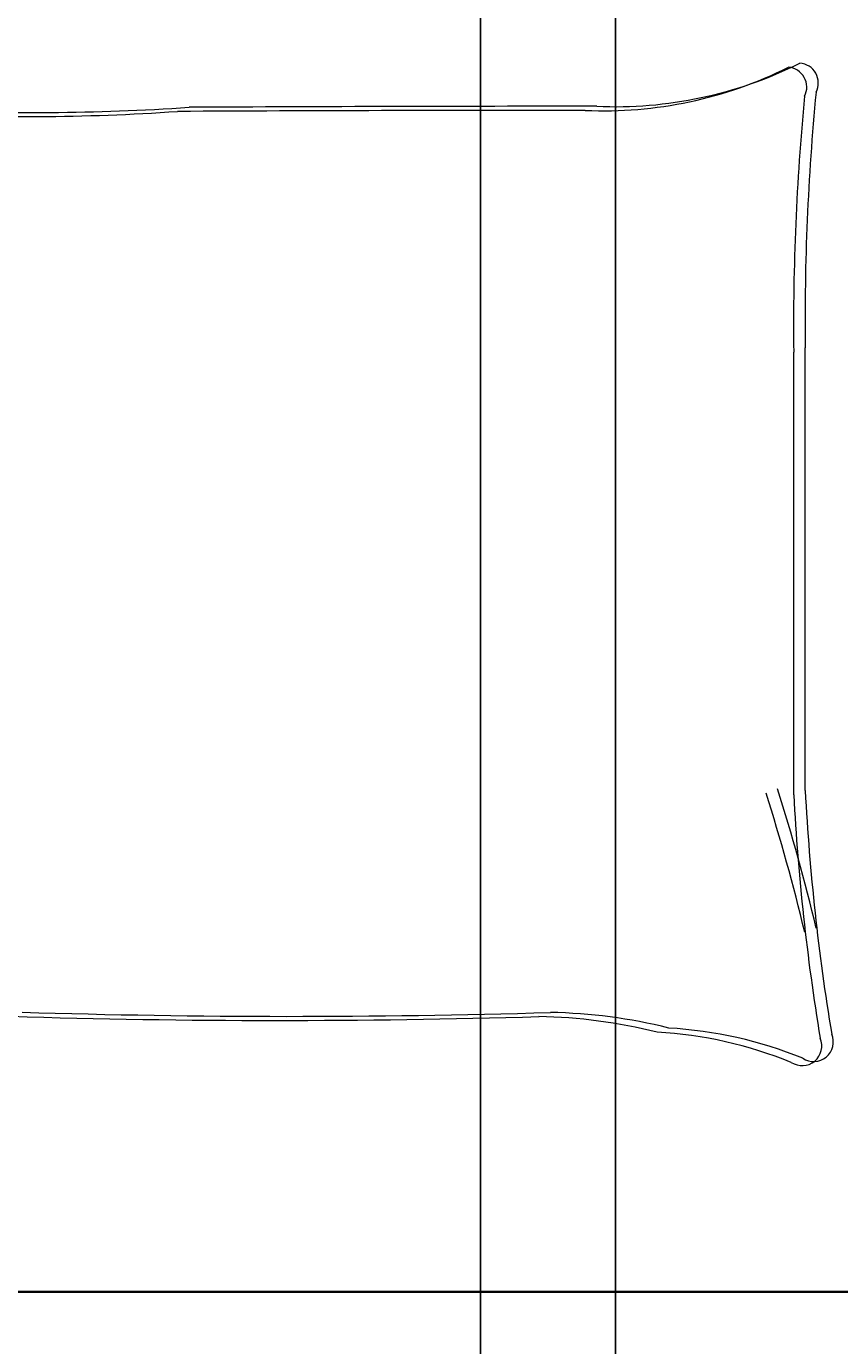
# Model space of a CAD drawing. Units: inches. Extents: x 1088 to 1703, y 668 to 1875.
# Tile 25 of 45: x 1484 to 1539, y 1416 to 1504. Entities that reach past the tile are written whole.
import ezdxf

# ---------------------------------------------------------------- set-up
doc = ezdxf.new("R2010")
doc.units = ezdxf.units.IN
for name, color, linetype, lineweight in [('A-ANNO-DIMS', 2, 'Continuous', 18), ('A-FURN', 8, 'Continuous', 13), ('A-WALL', 7, 'Continuous', 35)]:
    doc.layers.add(name, color=color, linetype=linetype, lineweight=lineweight)
doc.styles.get("Standard").update_dxf_attribs({"font": 'arial.ttf'})
doc.dimstyles.get("Standard").update_dxf_attribs({"dimtxt": 0.18, "dimasz": 0.18, "dimexe": 0.18, "dimexo": 0.0625, "dimgap": 0.09, "dimtad": 0, "dimtih": 1, "dimtoh": 1, "dimdec": 4, "dimzin": 0, "dimdsep": 46, "dimtxsty": 'Standard', "dimcen": 0.09, "dimadec": 0, "dimazin": 0, "dimtfac": 1, "dimtdec": 4, "dimtofl": 0, "dimtmove": 0, "dimatfit": 3, "dimfxl": 1, "dimtolj": 1, "dimtzin": 0, "dimarcsym": 0})

# ---------------------------------------------------------------- blocks, each defined once
blk = doc.blocks.new('BED-DOUBLE')
for p, q in [((95.003, 18.059), (95.003, 47.568)), ((95.77, 18.333), (95.77, 47.841))]:
    blk.add_line(p, q)
for centre, radius, start, end in [((82.321, 91.302), 27.652, 267.47136, 296.46809), ((83.088, 91.576), 27.652, 267.47136, 296.46809), ((94.554, 65.23), 1.322, 332.65876, 86.02002), ((95.32, 65.504), 1.322, 332.65876, 86.02002), ((254.489, 49.336), 159.496, 174.4998, 180.63509), ((255.256, 49.609), 159.496, 174.4998, 180.63509), ((43.537, 218.511), 155.251, 266.97912, 273.83645), ((44.303, 218.785), 155.251, 266.97912, 273.83645), ((81.308, -5405.342), 5469.019, 90.002168, 90.286887), ((82.075, -5405.068), 5469.019, 90.002168, 90.286887), ((-28.427, -20.646), 127.629, 13.38322, 17.70533), ((-27.661, -20.372), 127.629, 13.38322, 17.70533), ((240.775, 25.688), 145.971, 182.99578, 189.40907), ((241.542, 25.962), 145.971, 182.99578, 189.40907), ((61.445, 581.507), 578.221, 268.227709, 271.718541), ((78.111, -31.975), 35.527, 76.06484, 88.91125), ((60.679, 581.233), 578.221, 268.227709, 271.718541), ((77.344, -32.248), 35.527, 76.06484, 88.91125), ((84.25, -25.966), 28.247, 67.97508, 86.652), ((85.017, -25.693), 28.247, 67.97508, 86.652), ((95.57, 1.304), 1.306, 236.17358, 23.47814), ((96.337, 1.578), 1.306, 236.17358, 23.47814)]:
    blk.add_arc(centre, radius, start, end)
blk = doc.blocks.new('*D33')
at = {"layer": 'A-ANNO-DIMS', "color": 0, "lineweight": -2, "transparency": 16777216}
for p, q in [((1514.595, 1355.648), (1514.595, 1857.788)), ((1514.775, 1857.608), (1518.946, 1857.608)), ((1523.415, 1857.608), (1519.244, 1857.608)), ((1523.595, 1331.121), (1523.595, 1857.788))]:
    blk.add_line(p, q, dxfattribs=at)
at = {"layer": 'A-ANNO-DIMS', "color": 0, "transparency": 16777216}
for points in [[(1514.775, 1857.638), (1514.775, 1857.578), (1514.595, 1857.608)], [(1523.415, 1857.638), (1523.415, 1857.578), (1523.595, 1857.608)]]:
    blk.add_solid(points, dxfattribs=at)
at = {"layer": 'Defpoints', "color": 0, "transparency": 16777216}
for p in [(1523.595, 1857.608), (1514.595, 1355.585), (1523.595, 1331.058)]:
    blk.add_point(p, dxfattribs=at)
at = {"layer": 'A-ANNO-DIMS', "color": 0, "transparency": 16777216, "insert": (1519.095, 1857.608), "char_height": 0.18, "attachment_point": 5}
blk.add_mtext('\\A1;9', dxfattribs=at)

msp = doc.modelspace()

# ---------------------------------------------------------------- linework, layer by layer
at = {"layer": 'A-WALL'}
for p, q in [((1585.845, 1419.558), (1440.345, 1419.558)), ((1485.345, 1419.558), (1585.845, 1419.558))]:
    msp.add_line(p, q, dxfattribs=at)

# ---------------------------------------------------------------- block references
at = {"layer": 'A-FURN'}
msp.add_blockref('BED-DOUBLE', (1440.48, 1434.64), dxfattribs=at)

# ---------------------------------------------------------------- dimensions: what is measured, and where the dimension line sits
at = {"layer": 'A-ANNO-DIMS'}
dim = msp.add_linear_dim(base=(1523.595, 1857.608), p1=(1514.595, 1355.585), p2=(1523.595, 1331.058), dimstyle='Standard', override={"dimdec": 0, "dimlfac": 1, "dimrnd": 0, "dimzin": 0, "dimdsep": 46, "dimlunit": 2}, dxfattribs=at)
dim.commit()
dim.dimension.update_dxf_attribs({"geometry": '*D33', "text_midpoint": (1519.095, 1857.608)})

doc.saveas('drawing.dxf')
